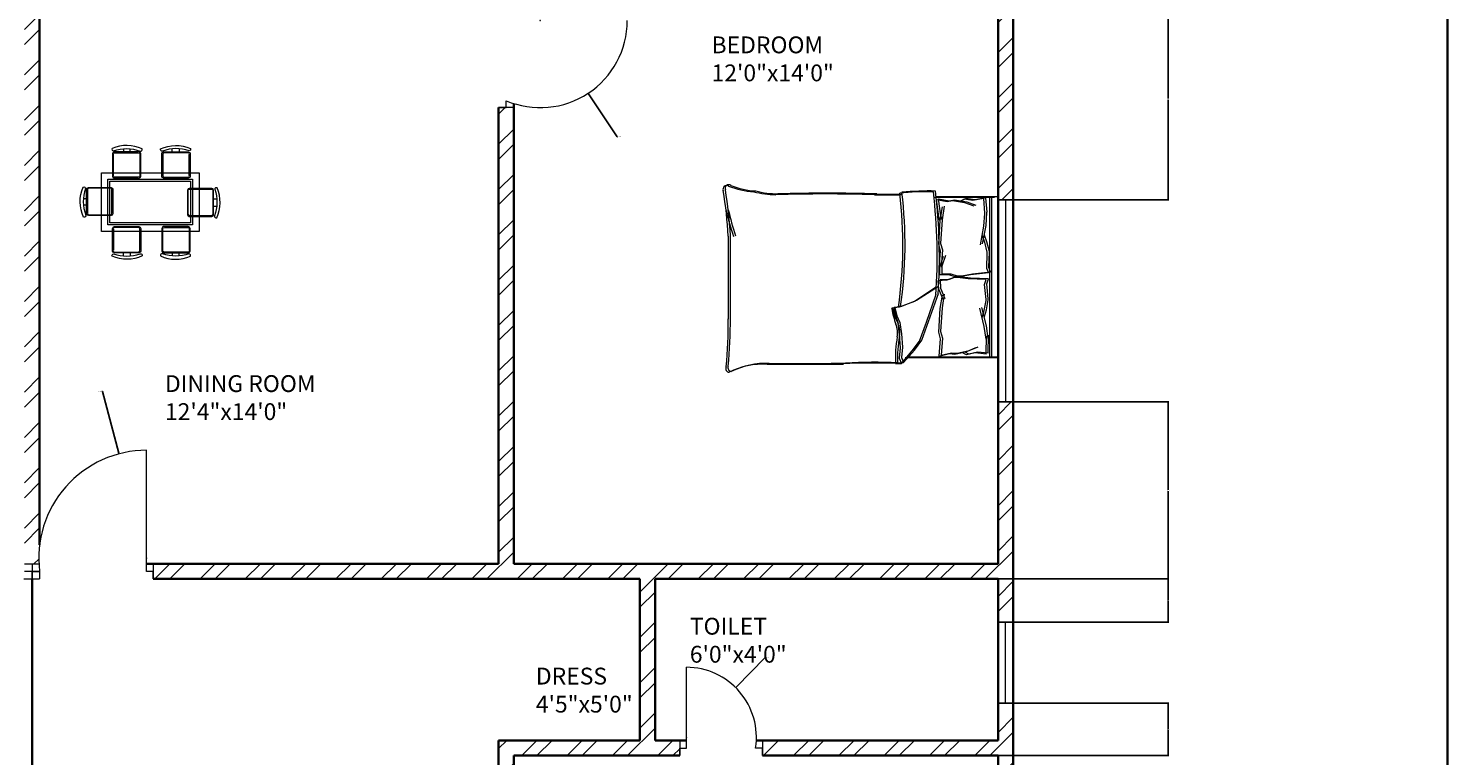
# Model space of a CAD drawing. Units: inches. Extents: x 392 to 1254, y 1207 to 2665.
# Tile 12 of 15: x 832 to 1254, y 1827 to 2043. Entities that reach past the tile are written whole.
import ezdxf

# ---------------------------------------------------------------- set-up
doc = ezdxf.new("R2010")
doc.units = ezdxf.units.IN
for name, color, linetype, lineweight in [('A-ANNO-DIMS', 2, 'Continuous', 18), ('A-ANNO-TTLB', 7, 'Continuous', 35), ('A-AREA-IDEN', 7, 'Continuous', 18), ('A-DOOR', 3, 'Continuous', 18), ('A-FURN', 8, 'Continuous', 13), ('A-GLAZ', 4, 'Continuous', 18), ('A-WALL', 7, 'Continuous', 35), ('A-WALL-PATT', 252, 'Continuous', 13)]:
    doc.layers.add(name, color=color, linetype=linetype, lineweight=lineweight)
doc.styles.get("Standard").update_dxf_attribs({"font": 'arial.ttf'})
doc.dimstyles.get("Standard").update_dxf_attribs({"dimtxt": 0.18, "dimasz": 0.18, "dimexe": 0.18, "dimexo": 0.0625, "dimgap": 0.09, "dimtad": 0, "dimtih": 1, "dimtoh": 1, "dimdec": 4, "dimzin": 0, "dimdsep": 46, "dimtxsty": 'Standard', "dimcen": 0.09, "dimadec": 0, "dimazin": 0, "dimtfac": 1, "dimtdec": 4, "dimtofl": 0, "dimtmove": 0, "dimatfit": 3, "dimfxl": 1, "dimtolj": 1, "dimtzin": 0, "dimarcsym": 0})

# ---------------------------------------------------------------- blocks, each defined once
blk = doc.blocks.new('BED-DOUBLE')
for p, q in [((3.47, 63.33), (3.47, 81.44)), ((3.48, 63.33), (3.48, 81.44)), ((3.7, 62.69), (3.7, 80.8)), ((3.7, 62.69), (3.7, 80.8)), ((51.27, 81.44), (51.27, 54.83)), ((51.27, 81.44), (51.27, 54.83)), ((51.49, 81.44), (51.49, 80.8)), ((51.49, 80.8), (51.49, 54.19)), ((51.49, 80.8), (51.49, 54.19)), ((3.47, 79.91), (51.27, 79.91)), ((3.48, 79.91), (51.27, 79.91)), ((3.7, 79.27), (51.49, 79.27)), ((3.7, 79.27), (51.49, 79.27)), ((3.89, 78.13), (4.47, 74.95)), ((3.89, 78.13), (4.47, 74.95)), ((3.9, 78.1), (8.18, 78.43)), ((3.9, 78.1), (8.18, 78.43)), ((4.12, 77.49), (4.7, 74.31)), ((4.12, 77.49), (4.7, 74.31)), ((4.13, 77.47), (8.41, 77.79)), ((4.13, 77.47), (8.41, 77.79)), ((8.18, 78.43), (8.28, 78.42)), ((8.18, 78.43), (8.28, 78.42)), ((8.28, 78.42), (12.11, 78.13)), ((8.28, 78.42), (12.11, 78.13)), ((8.41, 77.79), (8.51, 77.78)), ((8.41, 77.79), (8.51, 77.78)), ((8.51, 77.78), (12.34, 77.49)), ((8.51, 77.78), (12.34, 77.49)), ((12.11, 78.13), (17.6, 77.11)), ((12.11, 78.13), (17.6, 77.11)), ((12.34, 77.49), (17.83, 76.48)), ((12.34, 77.49), (17.83, 76.48)), ((14.85, 77.69), (16.88, 78.42)), ((14.85, 77.69), (16.88, 78.42)), ((15.08, 77.05), (17.11, 77.78)), ((15.08, 77.05), (17.11, 77.78)), ((16.88, 78.42), (19.77, 79.14)), ((16.88, 78.42), (19.77, 79.14)), ((17.11, 77.78), (20, 78.5)), ((17.11, 77.78), (20, 78.5)), ((19.77, 79.14), (20.09, 79.14)), ((19.77, 79.14), (20.09, 79.14)), ((20, 78.5), (20.32, 78.5)), ((20, 78.5), (20.32, 78.5)), ((20.09, 79.14), (24.54, 78.99)), ((20.09, 79.14), (24.54, 78.99)), ((20.32, 78.5), (24.77, 78.35)), ((20.32, 78.5), (24.77, 78.35)), ((24.54, 78.99), (25.98, 79.57)), ((24.54, 78.99), (25.98, 79.57)), ((24.77, 78.35), (26.21, 78.93)), ((24.77, 78.35), (26.21, 78.93)), ((25.98, 79.57), (26.56, 74.22)), ((25.98, 79.57), (26.56, 74.22)), ((26.21, 78.93), (26.79, 73.58)), ((26.21, 78.93), (26.79, 73.58)), ((27.98, 78.95), (27.73, 73.58)), ((27.98, 78.95), (27.73, 73.58)), ((28.21, 78.31), (27.96, 72.94)), ((28.21, 78.31), (27.96, 72.94)), ((29.46, 78.46), (27.98, 78.95)), ((29.46, 78.46), (27.98, 78.95)), ((29.68, 77.82), (28.21, 78.31)), ((29.68, 77.82), (28.21, 78.31)), ((33.88, 78.89), (29.46, 78.46)), ((33.88, 78.89), (29.46, 78.46)), ((34.11, 78.25), (29.68, 77.82)), ((34.11, 78.25), (29.68, 77.82)), ((34.2, 78.91), (33.88, 78.89)), ((34.2, 78.91), (33.88, 78.89)), ((34.43, 78.27), (34.11, 78.25)), ((34.43, 78.27), (34.11, 78.25)), ((37.14, 78.36), (34.2, 78.91)), ((37.14, 78.36), (34.2, 78.91)), ((37.36, 77.73), (34.43, 78.27)), ((37.36, 77.73), (34.43, 78.27)), ((41.91, 78.37), (36.49, 77.02)), ((41.91, 78.37), (36.5, 77.02)), ((42.14, 77.73), (36.72, 76.38)), ((42.14, 77.73), (36.72, 76.38)), ((39.2, 77.77), (37.14, 78.36)), ((39.2, 77.77), (37.14, 78.36)), ((39.43, 77.13), (37.36, 77.73)), ((39.43, 77.13), (37.36, 77.73)), ((45.71, 78.9), (41.91, 78.37)), ((45.71, 78.9), (41.91, 78.37)), ((45.94, 78.26), (42.14, 77.73)), ((45.94, 78.26), (42.14, 77.73)), ((50.11, 78.89), (44.71, 78.98)), ((44.71, 78.98), (45.71, 78.9)), ((50.11, 78.89), (44.71, 78.98)), ((44.71, 78.98), (45.71, 78.9)), ((50.34, 78.25), (44.94, 78.34)), ((44.94, 78.34), (45.94, 78.26)), ((50.34, 78.25), (44.94, 78.34)), ((44.94, 78.34), (45.94, 78.26)), ((50.11, 78.89), (49.73, 75.67)), ((50.11, 78.89), (49.73, 75.67)), ((50.34, 78.25), (49.96, 75.04)), ((50.34, 78.25), (49.96, 75.04)), ((4.47, 74.95), (4.04, 72.34)), ((4.47, 74.95), (4.04, 72.34)), ((4.04, 72.34), (4.62, 71.33)), ((4.04, 72.34), (4.62, 71.33)), ((4.7, 74.31), (4.27, 71.7)), ((4.7, 74.31), (4.27, 71.7)), ((4.47, 68.87), (5.05, 72.49)), ((4.47, 68.87), (5.05, 72.49)), ((4.7, 68.23), (5.28, 71.85)), ((4.7, 68.23), (5.28, 71.85)), ((5.05, 72.49), (6.06, 75.23)), ((5.05, 72.49), (6.06, 75.23)), ((5.28, 71.85), (6.29, 74.6)), ((5.28, 71.85), (6.29, 74.6)), ((26.56, 74.22), (27.14, 71.04)), ((26.56, 74.22), (27.14, 71.04)), ((26.79, 73.58), (27.37, 70.4)), ((26.79, 73.58), (27.37, 70.4)), ((27.73, 73.58), (27.35, 70.36)), ((27.73, 73.58), (27.35, 70.36)), ((27.96, 72.94), (27.58, 69.73)), ((27.96, 72.94), (27.58, 69.73)), ((49.31, 73.19), (48.13, 75.86)), ((49.31, 73.19), (48.13, 75.86)), ((49.54, 72.55), (48.36, 75.22)), ((49.54, 72.55), (48.36, 75.22)), ((50.11, 69.61), (49.31, 73.19)), ((50.11, 69.61), (49.31, 73.19)), ((50.34, 68.97), (49.54, 72.55)), ((50.34, 68.97), (49.54, 72.55)), ((49.73, 75.67), (50.33, 73.1)), ((49.73, 75.67), (50.33, 73.1)), ((50.33, 73.1), (49.81, 72.06)), ((50.33, 73.1), (49.81, 72.06)), ((49.96, 75.04), (50.56, 72.47)), ((49.96, 75.04), (50.56, 72.47)), ((50.56, 72.47), (50.04, 71.42)), ((50.56, 72.47), (50.04, 71.42)), ((4.27, 71.7), (4.85, 70.69)), ((4.27, 71.7), (4.85, 70.69)), ((4.76, 67.28), (4.47, 68.87)), ((4.76, 67.28), (4.47, 68.87)), ((4.99, 66.64), (4.7, 68.23)), ((4.99, 66.64), (4.7, 68.23)), ((27.14, 69.74), (26.56, 67.86)), ((27.14, 69.74), (26.56, 67.86)), ((26.56, 67.86), (26.56, 65.18)), ((26.56, 67.86), (26.56, 65.18)), ((27.37, 69.1), (26.79, 67.22)), ((27.37, 69.1), (26.79, 67.22)), ((27.14, 71.04), (27.14, 69.74)), ((27.14, 71.04), (27.14, 69.74)), ((27.35, 70.36), (27.44, 69.07)), ((27.35, 70.36), (27.44, 69.07)), ((27.37, 70.4), (27.37, 69.1)), ((27.37, 70.4), (27.37, 69.1)), ((27.44, 69.07), (28.13, 67.23)), ((27.44, 69.07), (28.13, 67.23)), ((27.58, 69.73), (27.66, 68.43)), ((27.58, 69.73), (27.66, 68.43)), ((27.66, 68.43), (28.36, 66.59)), ((27.66, 68.43), (28.36, 66.59)), ((49.92, 68.01), (50.11, 69.61)), ((49.92, 68.01), (50.11, 69.61)), ((50.7, 64.87), (49.92, 68.01)), ((50.7, 64.87), (49.92, 68.01)), ((50.15, 67.37), (50.34, 68.97)), ((50.15, 67.37), (50.34, 68.97)), ((4.18, 64.1), (4.76, 67.28)), ((4.18, 64.1), (4.76, 67.28)), ((9.28, 64.82), (4.18, 64.1)), ((9.28, 64.82), (4.18, 64.1)), ((4.41, 63.46), (4.99, 66.64)), ((4.41, 63.46), (4.99, 66.64)), ((9.51, 64.19), (4.41, 63.46)), ((9.51, 64.19), (4.41, 63.46)), ((6.38, 65.81), (10.41, 65.15)), ((6.38, 65.81), (10.41, 65.15)), ((6.61, 65.17), (10.64, 64.51)), ((6.61, 65.17), (10.64, 64.51)), ((10.41, 65.15), (9.28, 64.82)), ((10.41, 65.15), (9.28, 64.82)), ((10.64, 64.51), (9.51, 64.19)), ((10.64, 64.51), (9.51, 64.19)), ((10.41, 65.15), (17.42, 64.72)), ((10.41, 65.15), (17.42, 64.72)), ((10.64, 64.51), (17.65, 64.08)), ((10.64, 64.51), (17.65, 64.08)), ((17.42, 64.72), (19.38, 65.27)), ((17.42, 64.72), (19.38, 65.27)), ((17.65, 64.08), (19.61, 64.63)), ((17.65, 64.08), (19.61, 64.63)), ((19.38, 65.27), (24.52, 64.87)), ((19.38, 65.27), (24.52, 64.87)), ((19.61, 64.63), (24.74, 64.23)), ((19.61, 64.63), (24.74, 64.23)), ((24.1, 65.18), (20.96, 66.27)), ((24.1, 65.18), (20.96, 66.27)), ((24.33, 64.54), (21.19, 65.63)), ((24.33, 64.54), (21.19, 65.63)), ((26.56, 65.18), (24.1, 65.18)), ((26.56, 65.18), (24.1, 65.18)), ((26.79, 64.54), (24.33, 64.54)), ((26.79, 64.54), (24.33, 64.54)), ((26.79, 67.22), (26.79, 64.54)), ((26.79, 67.22), (26.79, 64.54)), ((28.13, 67.23), (28.3, 64.55)), ((28.13, 67.23), (28.3, 64.55)), ((28.3, 64.55), (30.75, 64.7)), ((28.3, 64.55), (30.75, 64.7)), ((28.36, 66.59), (28.53, 63.91)), ((28.36, 66.59), (28.53, 63.91)), ((28.53, 63.91), (30.98, 64.06)), ((28.53, 63.91), (30.98, 64.06)), ((30.26, 64.06), (34.45, 57.57)), ((30.26, 64.06), (34.45, 57.57)), ((30.49, 63.42), (34.68, 56.93)), ((30.49, 63.42), (34.68, 56.93)), ((30.75, 64.7), (33.82, 65.99)), ((30.75, 64.7), (33.82, 65.99)), ((30.98, 64.06), (34.05, 65.35)), ((30.98, 64.06), (34.05, 65.35)), ((40.64, 61.13), (32.31, 64.06)), ((40.64, 61.13), (32.31, 64.06)), ((40.87, 60.49), (32.53, 63.42)), ((40.87, 60.49), (32.53, 63.42)), ((32.56, 65.81), (36.6, 65.15)), ((32.56, 65.81), (36.6, 65.15)), ((32.79, 65.17), (36.82, 64.51)), ((32.79, 65.17), (36.82, 64.51)), ((36.6, 65.15), (43.61, 64.72)), ((36.6, 65.15), (43.61, 64.72)), ((36.82, 64.51), (43.83, 64.08)), ((36.82, 64.51), (43.83, 64.08)), ((43.61, 64.72), (45.57, 65.27)), ((43.61, 64.72), (45.57, 65.27)), ((43.83, 64.08), (45.79, 64.63)), ((43.83, 64.08), (45.79, 64.63)), ((45.57, 65.27), (50.7, 64.87)), ((45.57, 65.27), (50.7, 64.87)), ((45.79, 64.63), (50.93, 64.23)), ((45.79, 64.63), (50.93, 64.23)), ((50.93, 64.23), (50.15, 67.37)), ((50.93, 64.23), (50.15, 67.37)), ((46.22, 59.11), (40.64, 61.13)), ((46.22, 59.11), (40.64, 61.13)), ((46.45, 58.47), (40.87, 60.49)), ((46.45, 58.47), (40.87, 60.49)), ((49.16, 56.95), (46.22, 59.11)), ((49.16, 56.95), (46.22, 59.11)), ((34.45, 57.57), (36.15, 53.08)), ((34.45, 57.57), (36.15, 53.08)), ((34.68, 56.93), (36.38, 52.44)), ((34.68, 56.93), (36.38, 52.44)), ((49.39, 56.31), (46.45, 58.47)), ((49.39, 56.31), (46.45, 58.47)), ((52.87, 53.7), (49.16, 56.95)), ((52.87, 53.7), (49.16, 56.95)), ((53.1, 53.06), (49.39, 56.31)), ((53.1, 53.06), (49.39, 56.31)), ((36.15, 53.08), (36.46, 51.07)), ((36.15, 53.08), (36.46, 51.07)), ((36.38, 52.44), (36.69, 50.43)), ((36.38, 52.44), (36.69, 50.43)), ((36.46, 51.07), (38.94, 51.68)), ((36.46, 51.07), (38.94, 51.68)), ((36.69, 50.43), (39.17, 51.05)), ((36.69, 50.43), (39.17, 51.05)), ((38.94, 51.68), (40.95, 52.61)), ((38.94, 51.68), (40.95, 52.61)), ((39.17, 51.05), (41.18, 51.97)), ((39.17, 51.05), (41.18, 51.97)), ((40.95, 52.61), (44.36, 53.08)), ((40.95, 52.61), (44.36, 53.08)), ((41.18, 51.97), (44.59, 52.44)), ((41.18, 51.97), (44.59, 52.44)), ((44.36, 53.08), (48.23, 53.39)), ((44.36, 53.08), (48.23, 53.39)), ((44.59, 52.44), (48.46, 52.75)), ((44.59, 52.44), (48.46, 52.75)), ((48.23, 53.39), (51.33, 53.08)), ((48.23, 53.39), (51.33, 53.08)), ((48.46, 52.75), (51.56, 52.44)), ((48.46, 52.75), (51.56, 52.44)), ((51.33, 53.08), (52.87, 53.7)), ((51.33, 53.08), (52.87, 53.7)), ((51.56, 52.44), (53.1, 53.06)), ((51.56, 52.44), (53.1, 53.06)), ((52.95, 51.95), (52.87, 53.7, 3.87)), ((52.95, 51.95), (52.87, 53.7, 3.87)), ((53.18, 51.31), (53.1, 53.06, 3.87)), ((53.18, 51.31), (53.1, 53.06, 3.87)), ((15.06, 2.2), (39.68, 2.2)), ((15.06, 2.2), (39.68, 2.2)), ((15.29, 1.56), (39.91, 1.56)), ((15.29, 1.56), (39.91, 1.56))]:
    blk.add_line(p, q)
for centre, radius, start, end in [((21.36, -100.61), 164.97, 86.0865, 96.7821), ((21.36, -100.61), 164.97, 86.0865, 96.7821), ((21.59, -101.25), 164.97, 86.0865, 96.7821), ((21.59, -101.25), 164.97, 86.0865, 96.7821), ((85.16, 61.35), 83.31, 178.7218, 185.604), ((85.16, 61.35), 83.31, 178.7218, 185.604), ((85.39, 60.71), 83.31, 178.7218, 185.604), ((85.39, 60.71), 83.31, 178.7218, 185.604), ((17.76, -74.87), 129.02, 81.7845, 96.9006), ((17.76, -74.87), 129.02, 81.7845, 96.9006), ((17.98, -75.51), 129.02, 81.7845, 96.9006), ((17.98, -75.51), 129.02, 81.7845, 96.9006), ((-167.31, 50.27), 170.11, 358.4762, 1.0082), ((-167.31, 50.27), 170.11, 358.4762, 1.0082), ((-167.08, 49.63), 170.11, 358.4762, 1.0082), ((-167.08, 49.63), 170.11, 358.4762, 1.0082), ((36.64, 51), 0.185, 160.2464, 271.1377), ((36.64, 51), 0.185, 160.2464, 271.1377), ((31.15, 79.96), 29.65, 280.6617, 289.8806), ((31.15, 79.96), 29.65, 280.6617, 289.8806), ((31.38, 79.32), 29.65, 280.6617, 289.8806), ((31.38, 79.32), 29.65, 280.6617, 289.8806), ((43.74, 46.38), 6.22, 78.6608, 113.7384), ((43.74, 46.38), 6.22, 78.6608, 113.7384), ((43.97, 45.74), 6.22, 78.6608, 113.7384), ((43.97, 45.74), 6.22, 78.6608, 113.7384), ((51.33, 88.1), 36.18, 259.8763, 272.5657), ((51.33, 88.1), 36.18, 259.8763, 272.5657), ((51.56, 87.46), 36.18, 259.8763, 272.5657), ((51.56, 87.46), 36.18, 259.8763, 272.5657), ((182.27, 45.13), 129.5, 176.9791, 183.8365), ((182.27, 45.13), 129.5, 176.9791, 183.8365), ((182.49, 44.49), 129.5, 176.9791, 183.8365), ((182.49, 44.49), 129.5, 176.9791, 183.8365), ((36.86, 50.36), 0.185, 160.2464, 271.1377), ((36.86, 50.36), 0.185, 160.2464, 271.1377), ((484.82, 30.83), 482.31, 178.2277, 181.7185), ((484.82, 30.83), 482.31, 178.2277, 181.7185), ((485.05, 30.19), 482.31, 178.2277, 181.7185), ((485.05, 30.19), 482.31, 178.2277, 181.7185), ((-4508.74, 13.62), 4561.86, 0.00217, 0.28689), ((-4508.74, 13.62), 4561.86, 0.00217, 0.28689), ((-4508.51, 12.98), 4561.86, 0.00217, 0.28689), ((-4508.52, 12.98), 4561.86, 0.00217, 0.28689), ((-26.9, 16.93), 29.63, 346.0648, 358.9113), ((-26.9, 16.93), 29.63, 346.0648, 358.9113), ((-26.67, 16.29), 29.63, 346.0648, 358.9113), ((-26.67, 16.29), 29.63, 346.0648, 358.9113), ((76.16, 12.78), 23.07, 177.4714, 206.4681), ((76.16, 12.78), 23.07, 177.4714, 206.4681), ((76.39, 12.14), 23.07, 177.4714, 206.4681), ((76.39, 12.14), 23.07, 177.4714, 206.4681), ((-21.66, 11.17), 23.56, 337.9751, 356.652), ((-21.66, 11.17), 23.56, 337.9751, 356.652), ((-21.43, 10.53), 23.56, 337.9751, 356.652), ((-21.43, 10.53), 23.56, 337.9751, 356.652), ((1.09, 1.72), 1.09, 146.1736, 293.4781), ((1.09, 1.72), 1.09, 146.1736, 293.4781), ((1.32, 1.09), 1.09, 146.1736, 293.4781), ((1.32, 1.09), 1.09, 146.1736, 293.4781), ((21.43, -119.39), 121.76, 92.9958, 99.4091), ((21.43, -119.39), 121.76, 92.9958, 99.4091), ((21.66, -120.03), 121.76, 92.9958, 99.4091), ((21.65, -120.03), 121.76, 92.9958, 99.4091), ((-17.22, 105.15), 106.46, 283.3832, 287.7053), ((-17.22, 105.15), 106.46, 283.3832, 287.7053), ((-16.99, 104.52), 106.46, 283.3832, 287.7053), ((-16.99, 104.52), 106.46, 283.3832, 287.7053), ((41.15, -130.83), 133.04, 84.4998, 90.6351), ((41.15, -130.83), 133.04, 84.4998, 90.6351), ((41.38, -131.47), 133.04, 84.4998, 90.6351), ((41.38, -131.47), 133.04, 84.4998, 90.6351), ((54.41, 2.57), 1.1, 242.6588, 356.02), ((54.41, 2.57), 1.1, 242.6588, 356.02), ((54.64, 1.93), 1.1, 242.6588, 356.02), ((54.64, 1.93), 1.1, 242.6588, 356.02)]:
    blk.add_arc(centre, radius, start, end)
blk = doc.blocks.new('TABLE-DINING-RECT')
for points in [[(0, 17.41), (29.01, 17.41), (29.01, 0), (0, 0)], [(0, 17.41), (29.01, 17.41), (29.01, 0), (0, 0)], [(1.93, 15.47), (27.08, 15.47), (27.08, 1.93), (1.93, 1.93)], [(1.93, 15.47), (27.08, 15.47), (27.08, 1.93), (1.93, 1.93)], [(2.51, 14.89), (26.5, 14.89), (26.5, 2.51), (2.51, 2.51)], [(2.51, 14.89), (26.5, 14.89), (26.5, 2.51), (2.51, 2.51)]]:
    blk.add_lwpolyline(points, close=True)
blk = doc.blocks.new('WIN-60-A')
for p, q in [((0, 60), (4.5, 60)), ((4.5, 60), (2.25, 60)), ((2.25, 60), (2.25, 0)), ((2.25, 0), (0, 0)), ((0, 0), (4.5, 0))]:
    blk.add_line(p, q)
blk = doc.blocks.new('WIN-24-B')
for p, q in [((2.25, 24), (0, 24)), ((0, 24), (4.5, 24)), ((2.25, 0), (2.25, 24)), ((0, 0), (4.5, 0)), ((4.5, 0), (2.25, 0))]:
    blk.add_line(p, q)
blk = doc.blocks.new('*D32')
at = {"layer": 'A-ANNO-DIMS', "color": 0, "lineweight": -2, "transparency": 16777216}
for p, q in [((1120.34, 1842.92), (1171.06, 1842.92)), ((1170.88, 1842.74), (1170.88, 1835.29)), ((1170.88, 1827.48), (1170.88, 1834.93)), ((1120.34, 1827.3), (1171.06, 1827.3))]:
    blk.add_line(p, q, dxfattribs=at)
at = {"layer": 'A-ANNO-DIMS', "color": 0, "transparency": 16777216}
for points in [[(1170.85, 1842.74), (1170.91, 1842.74), (1170.88, 1842.92)], [(1170.85, 1827.48), (1170.91, 1827.48), (1170.88, 1827.3)]]:
    blk.add_solid(points, dxfattribs=at)
at = {"layer": 'Defpoints', "color": 0, "transparency": 16777216}
for p in [(1120.28, 1842.92), (1170.88, 1842.92), (1120.28, 1827.3)]:
    blk.add_point(p, dxfattribs=at)
at = {"layer": 'A-ANNO-DIMS', "color": 0, "transparency": 16777216, "insert": (1170.88, 1835.11), "char_height": 0.18, "attachment_point": 5}
blk.add_mtext('\\A1;15.624', dxfattribs=at)
blk = doc.blocks.new('*D33')
at = {"layer": 'A-ANNO-DIMS', "color": 0, "lineweight": -2, "transparency": 16777216}
for p, q in [((1120.34, 1932.46), (1171.06, 1932.46)), ((1170.88, 1932.28), (1170.88, 1906.31)), ((1170.88, 1879.98), (1170.88, 1905.94)), ((1120.34, 1879.8), (1171.06, 1879.8))]:
    blk.add_line(p, q, dxfattribs=at)
at = {"layer": 'A-ANNO-DIMS', "color": 0, "transparency": 16777216}
for points in [[(1170.85, 1932.28), (1170.91, 1932.28), (1170.88, 1932.46)], [(1170.85, 1879.98), (1170.91, 1879.98), (1170.88, 1879.8)]]:
    blk.add_solid(points, dxfattribs=at)
at = {"layer": 'Defpoints', "color": 0, "transparency": 16777216}
for p in [(1120.28, 1932.46), (1170.88, 1932.46), (1120.28, 1879.8)]:
    blk.add_point(p, dxfattribs=at)
at = {"layer": 'A-ANNO-DIMS', "color": 0, "transparency": 16777216, "insert": (1170.88, 1906.13), "char_height": 0.18, "attachment_point": 5}
blk.add_mtext('\\A1;52.66', dxfattribs=at)
blk = doc.blocks.new('*D40')
at = {"layer": 'A-ANNO-DIMS', "color": 0, "lineweight": -2, "transparency": 16777216}
for p, q in [((1120.34, 2052.3), (1171.06, 2052.3)), ((1170.88, 2052.12), (1170.88, 2022.56)), ((1170.88, 1992.64), (1170.88, 2022.19)), ((1120.34, 1992.46), (1171.06, 1992.46))]:
    blk.add_line(p, q, dxfattribs=at)
at = {"layer": 'A-ANNO-DIMS', "color": 0, "transparency": 16777216}
for points in [[(1170.85, 2052.12), (1170.91, 2052.12), (1170.88, 2052.3)], [(1170.85, 1992.64), (1170.91, 1992.64), (1170.88, 1992.46)]]:
    blk.add_solid(points, dxfattribs=at)
at = {"layer": 'Defpoints', "color": 0, "transparency": 16777216}
for p in [(1120.28, 2052.3), (1120.28, 1992.46), (1170.88, 1992.46)]:
    blk.add_point(p, dxfattribs=at)
at = {"layer": 'A-ANNO-DIMS', "color": 0, "transparency": 16777216, "insert": (1170.88, 2022.38), "char_height": 0.18, "attachment_point": 5}
blk.add_mtext('\\A1;59.84', dxfattribs=at)
blk = doc.blocks.new('*D41')
at = {"layer": 'A-ANNO-DIMS', "color": 0, "lineweight": -2, "transparency": 16777216}
for p, q in [((1120.34, 1879.8), (1171.06, 1879.8)), ((1170.88, 1879.62), (1170.88, 1873.54)), ((1170.88, 1867.1), (1170.88, 1873.18)), ((1120.34, 1866.92), (1171.06, 1866.92))]:
    blk.add_line(p, q, dxfattribs=at)
at = {"layer": 'A-ANNO-DIMS', "color": 0, "transparency": 16777216}
for points in [[(1170.85, 1879.62), (1170.91, 1879.62), (1170.88, 1879.8)], [(1170.85, 1867.1), (1170.91, 1867.1), (1170.88, 1866.92)]]:
    blk.add_solid(points, dxfattribs=at)
at = {"layer": 'Defpoints', "color": 0, "transparency": 16777216}
for p in [(1120.28, 1879.8), (1120.28, 1866.92), (1170.88, 1866.92)]:
    blk.add_point(p, dxfattribs=at)
at = {"layer": 'A-ANNO-DIMS', "color": 0, "transparency": 16777216, "insert": (1170.88, 1873.36), "char_height": 0.18, "attachment_point": 5}
blk.add_mtext('\\A1;12.876', dxfattribs=at)
blk = doc.blocks.new('*D84')
at = {"layer": 'A-ANNO-DIMS', "color": 0, "lineweight": -2, "transparency": 16777216}
for p, q in [((853.76, 1935.56), (853.94, 1935.56)), ((853.94, 1935.56), (858.83, 1917.15)), ((867, 1885.99), (867.18, 1885.99)), ((867.09, 1885.9), (867.09, 1886.08))]:
    blk.add_line(p, q, dxfattribs=at)
at = {"layer": 'A-ANNO-DIMS', "color": 0, "transparency": 16777216}
blk.add_solid([(858.86, 1917.16), (858.8, 1917.14), (858.87, 1916.97)], dxfattribs=at)
at = {"layer": 'Defpoints', "color": 0, "transparency": 16777216}
for p in [(858.87, 1916.97), (867.09, 1885.99)]:
    blk.add_point(p, dxfattribs=at)
at = {"layer": 'A-ANNO-DIMS', "color": 0, "transparency": 16777216, "insert": (853.21, 1935.56), "char_height": 0.18, "attachment_point": 5}
blk.add_mtext('\\A1;R32.054', dxfattribs=at)
blk = doc.blocks.new('*D96')
at = {"layer": 'A-ANNO-DIMS', "color": 0, "lineweight": -2, "transparency": 16777216}
for p, q in [((984.08, 2045.75), (984.26, 2045.75)), ((984.17, 2045.66), (984.17, 2045.84)), ((1006.98, 2011.23), (998.53, 2024.02)), ((1007.16, 2011.23), (1006.98, 2011.23))]:
    blk.add_line(p, q, dxfattribs=at)
at = {"layer": 'A-ANNO-DIMS', "color": 0, "transparency": 16777216}
blk.add_solid([(998.55, 2024.04), (998.5, 2024.01), (998.43, 2024.17)], dxfattribs=at)
at = {"layer": 'Defpoints', "color": 0, "transparency": 16777216}
for p in [(984.17, 2045.75), (998.43, 2024.17)]:
    blk.add_point(p, dxfattribs=at)
at = {"layer": 'A-ANNO-DIMS', "color": 0, "transparency": 16777216, "insert": (1007.71, 2011.23), "char_height": 0.18, "attachment_point": 5}
blk.add_mtext('\\A1;R25.864', dxfattribs=at)
blk = doc.blocks.new('*D102')
at = {"layer": 'A-ANNO-DIMS', "color": 0, "lineweight": -2, "transparency": 16777216}
for p, q in [((1051.03, 1856.44), (1042.37, 1847.67)), ((1051.21, 1856.44), (1051.03, 1856.44)), ((1027.53, 1832.72), (1027.71, 1832.72)), ((1027.62, 1832.63), (1027.62, 1832.81))]:
    blk.add_line(p, q, dxfattribs=at)
at = {"layer": 'A-ANNO-DIMS', "color": 0, "transparency": 16777216}
blk.add_solid([(1042.35, 1847.69), (1042.4, 1847.65), (1042.25, 1847.54)], dxfattribs=at)
at = {"layer": 'Defpoints', "color": 0, "transparency": 16777216}
for p in [(1042.25, 1847.54), (1027.62, 1832.72)]:
    blk.add_point(p, dxfattribs=at)
at = {"layer": 'A-ANNO-DIMS', "color": 0, "transparency": 16777216, "insert": (1051.76, 1856.44), "char_height": 0.18, "attachment_point": 5}
blk.add_mtext('\\A1;R20.826', dxfattribs=at)

msp = doc.modelspace()

# ---------------------------------------------------------------- hatches: boundary and pattern name
at = {"layer": 'A-WALL-PATT'}
h = msp.add_hatch(dxfattribs=at)
h.set_pattern_fill('ANSI32', color=256)
h.paths.add_polyline_path([(579.5309, 2227.0453), (579.5309, 2229.2953), (541.2807, 2229.2953), (541.2807, 2182.3091), (545.7807, 2182.3091), (545.7807, 2224.7953), (579.5309, 2224.7953)])
h.paths.add_polyline_path([(655.4442, 2229.2953), (627.5309, 2229.2953), (627.5309, 2224.7953), (655.4442, 2224.7953), (655.4442, 2227.0453)])
h.paths.add_polyline_path([(703.0758, 2229.2953), (678.5257, 2229.2953), (678.5257, 2227.0453), (678.5257, 2224.7953), (689.7807, 2224.7953), (689.7807, 2158.6973), (694.2807, 2158.6973), (694.2807, 2224.7953), (703.0758, 2224.7953)])
h.paths.add_polyline_path([(768.5767, 2229.2953), (727.0758, 2229.2953), (727.0758, 2224.7953), (742.2807, 2224.7953), (742.2807, 2128.7953), (694.2807, 2128.7953), (694.2807, 2134.0554), (689.7807, 2134.0554), (689.7807, 2090.2854), (694.2807, 2090.2854), (694.2807, 2124.2953), (742.2807, 2124.2953), (742.2807, 2052.2953), (795.2124, 2052.2953), (795.2124, 2054.5453), (795.2124, 2056.7953), (746.7807, 2056.7953), (746.7807, 2224.7953), (768.5767, 2224.7953)])
h.paths.add_polyline_path([(867.5089, 2229.2953), (804.5767, 2229.2953), (804.5767, 2224.7953), (830.7807, 2224.7953), (830.7807, 2056.7953), (826.9066, 2056.7953), (826.9066, 2052.2953), (830.7807, 2052.2953), (830.7807, 1886.6777, -0.01766664), (830.8602, 1884.2953), (835.0818, 1884.2953, -0.04411348), (835.2807, 1889.9369), (835.2807, 2052.2953), (839.418, 2052.2953), (839.418, 2056.7953), (835.2807, 2056.7953), (835.2807, 2224.7953), (867.5089, 2224.7953)])
h.paths.add_polyline_path([(939.8604, 2229.2953), (903.5089, 2229.2953), (903.5089, 2227.0453), (903.5089, 2224.7953), (919.2807, 2224.7953), (919.2807, 2056.7953), (870.6499, 2056.7953), (870.6499, 2052.2953), (923.7807, 2052.2953), (923.7807, 2124.2953), (971.7807, 2124.2953), (971.7807, 2089.7112), (974.0307, 2089.7112), (976.2807, 2089.7112), (976.2807, 2133.56), (974.0307, 2133.56), (971.7807, 2133.56), (971.7807, 2128.7953), (923.7807, 2128.7953), (923.7807, 2224.7953), (939.8604, 2224.7953)])
h.paths.add_polyline_path([(1124.7807, 2229.2953), (1009.403, 2229.2953), (1009.403, 2224.7953), (1120.2807, 2224.7953), (1120.2807, 2184.7605), (1124.7807, 2184.7605)])
h.paths.add_polyline_path([(1124.7807, 2124.7605), (1120.2807, 2124.7605), (1120.2807, 2056.7953), (976.2807, 2056.7953), (976.2807, 2061.471), (971.7807, 2061.471), (971.7807, 2047.7483), (974.0307, 2047.7483), (976.2807, 2047.7483), (976.2807, 2052.2953), (1120.2807, 2052.2953), (1120.2807, 1992.457), (1124.7807, 1992.457)])
h.paths.add_polyline_path([(1124.7807, 1932.457), (1122.5307, 1932.457), (1120.2807, 1932.457), (1120.2807, 1884.2953), (976.2807, 1884.2953), (976.2807, 2019.9536), (971.7807, 2019.9536), (971.7807, 1884.2953), (869.0911, 1884.2953), (869.0911, 1879.7953), (971.7807, 1879.7953), (1013.7807, 1879.7953), (1013.7807, 1831.7953), (971.7807, 1831.7953), (971.7807, 1822.3831), (974.0307, 1822.3831), (976.2807, 1822.3831), (976.2807, 1827.2953), (1013.7807, 1827.2953), (1025.6191, 1827.2953), (1025.6191, 1829.5453), (1025.6191, 1831.7953), (1018.2807, 1831.7953), (1018.2807, 1879.7953), (1120.2807, 1879.7953), (1120.2807, 1866.9192), (1124.7807, 1866.9192)])
h.paths.add_polyline_path([(1124.7807, 1842.9192), (1122.5307, 1842.9192), (1120.2807, 1842.9192), (1120.2807, 1831.7953), (1050.2021, 1831.7953), (1050.2021, 1827.2953), (1120.2807, 1827.2953), (1120.2807, 1781.4559), (1124.7807, 1781.4559)])
h.paths.add_polyline_path([(976.2807, 1790.8718), (971.7807, 1790.8718), (971.7807, 1648.3339), (976.2807, 1648.3339), (976.2807, 1654.7953), (1120.2807, 1654.7953), (1120.2807, 1626.3807), (1124.7807, 1626.3807), (1124.7807, 1721.4559), (1120.2807, 1721.4559), (1120.2807, 1659.2953), (976.2807, 1659.2953)])
h.paths.add_polyline_path([(1124.7807, 1566.3807), (1120.2807, 1566.3807), (1120.2807, 1486.7953), (1101.07, 1486.7953), (1101.07, 1482.2953), (1124.7807, 1482.2953)])
h.paths.add_polyline_path([(1041.07, 1484.5453), (1041.07, 1486.7953), (1006.2807, 1486.7953), (1006.2807, 1484.5453), (1006.2807, 1482.2953), (1041.07, 1482.2953)])
h.paths.add_polyline_path([(976.2807, 1617.5497), (974.0307, 1617.5497), (971.7807, 1617.5497), (971.7807, 1599.2953), (965.8041, 1599.2953), (965.8041, 1594.7953), (971.7807, 1594.7953), (971.7807, 1486.7953), (954.1249, 1486.7953), (954.1249, 1482.2953), (981.5717, 1482.2953), (981.5717, 1484.5453), (981.5717, 1486.7953), (976.2807, 1486.7953)])
h.paths.add_polyline_path([(930.1249, 1486.7953), (887.7807, 1486.7953), (887.7807, 1594.7953), (941.9141, 1594.7953), (941.9141, 1597.0453), (941.9141, 1599.2953), (887.7807, 1599.2953), (887.7807, 1659.2953), (863.5916, 1659.2953), (863.5916, 1654.7953), (883.2807, 1654.7953), (883.2807, 1438.7953), (782.7807, 1438.7953), (782.7807, 1486.7953), (782.7807, 1654.7953), (800.1309, 1654.7953), (800.1309, 1657.0453), (800.1309, 1659.2953), (778.2807, 1659.2953), (778.2807, 1599.2953), (721.7333, 1599.2953), (721.7333, 1597.0453), (721.7333, 1594.7953), (778.2807, 1594.7953), (778.2807, 1486.7953), (729.598, 1486.7953), (729.598, 1482.2953), (753.2885, 1482.2953), (753.2885, 1410.2953), (922.9852, 1410.2953), (922.9852, 1482.2953), (930.1249, 1482.2953)])
h.paths.add_polyline_path([(918.4852, 1482.2953), (918.4852, 1414.7953), (757.7885, 1414.7953), (757.7885, 1482.2953), (778.2807, 1482.2953), (778.2807, 1434.2953), (782.7807, 1434.2953), (887.7807, 1434.2953), (887.7807, 1438.7953), (887.7807, 1482.2953)], flags=16)
h.paths.add_polyline_path([(694.2807, 1594.7953), (700.4169, 1594.7953), (700.4169, 1597.0453), (700.4169, 1599.2953), (694.2807, 1599.2953), (694.2807, 1617.7503), (692.0307, 1617.7503), (689.7807, 1617.7503), (689.7807, 1486.7953), (682.7672, 1486.7953), (682.7672, 1482.2953), (705.598, 1482.2953), (705.598, 1484.5453), (705.598, 1486.7953), (694.2807, 1486.7953)])
h.paths.add_polyline_path([(545.7807, 1654.7953), (689.7807, 1654.7953), (689.7807, 1649.7691), (694.2807, 1649.7691), (694.2807, 1789.3981), (692.0307, 1789.3981), (689.7807, 1789.3981), (689.7807, 1659.2953), (545.7807, 1659.2953), (545.7807, 1714.4681), (543.5307, 1714.4681), (541.2807, 1714.4681), (541.2807, 1482.2953), (567.0628, 1482.2953), (567.0628, 1484.5453), (567.0628, 1486.7953), (545.7807, 1486.7953)])
h.paths.add_polyline_path([(545.7807, 1827.2953), (620.2247, 1827.2953), (620.2247, 1829.5453), (620.2247, 1831.7953), (545.7807, 1831.7953), (545.7807, 1846.8518), (541.2807, 1846.8518), (541.2807, 1774.4681), (545.7807, 1774.4681)])
h.paths.add_polyline_path([(797.0944, 1884.2953), (694.2807, 1884.2953), (694.2807, 2019.0288), (692.0307, 2019.0288), (689.7807, 2019.0288), (689.7807, 1884.2953), (545.7807, 1884.2953), (545.7807, 1951.8244), (541.2807, 1951.8244), (541.2807, 1870.8518), (543.5307, 1870.8518), (545.7807, 1870.8518), (545.7807, 1879.7953), (647.7807, 1879.7953), (647.7807, 1831.7953), (642.6413, 1831.7953), (642.6413, 1827.2953), (652.2807, 1827.2953), (689.7807, 1827.2953), (689.7807, 1821.0531), (694.2807, 1821.0531), (694.2807, 1831.7953), (652.2807, 1831.7953), (652.2807, 1879.7953), (797.0944, 1879.7953), (797.0944, 1882.0453)])
h.paths.add_polyline_path([(545.7807, 2122.3091), (541.2807, 2122.3091), (541.2807, 2011.8244), (543.5307, 2011.8244), (545.7807, 2011.8244), (545.7807, 2052.2953), (689.7807, 2052.2953), (689.7807, 2048.2048), (694.2807, 2048.2048), (694.2807, 2061.3129), (692.0307, 2061.3129), (689.7807, 2061.3129), (689.7807, 2056.7953), (545.7807, 2056.7953)])

# ---------------------------------------------------------------- linework, layer by layer
at = {"layer": 'A-ANNO-TTLB'}
msp.add_lwpolyline([(391.939, 2664.8979), (1253.97, 2664.8979), (1253.97, 1207.2611), (391.939, 1207.2611)], close=True, dxfattribs=at)
at = {"layer": 'A-DOOR'}
for p, q in [((974.0307, 2019.9536), (974.0307, 2021.9536)), ((976.2807, 2019.9536), (971.7807, 2019.9536)), ((971.7807, 2019.9536), (974.0307, 2019.9536)), ((867.0911, 1882.0453), (867.0911, 1918.0453)), ((830.7807, 1884.2953), (835.0818, 1884.2953)), ((833.0352, 1884.2953), (833.0352, 1879.7953)), ((869.0911, 1884.2953), (869.0911, 1879.7953)), ((830.5499, 1879.7953), (835.2807, 1879.7953)), ((833.0352, 1882.0453), (830.7807, 1882.0453)), ((833.0352, 1879.7953), (833.0352, 1882.0453)), ((833.0352, 1882.0453), (835.2807, 1882.0453)), ((835.2807, 1882.0453), (833.0352, 1882.0453)), ((835.2807, 1882.0453), (835.2807, 1879.7953)), ((869.0911, 1882.0453), (867.0911, 1882.0453)), ((869.0911, 1879.7953), (869.0911, 1882.0453)), ((1027.6191, 1829.5453), (1027.6191, 1853.5453)), ((1025.6191, 1831.7953), (1025.6191, 1827.2953)), ((1050.2021, 1831.7953), (1050.2021, 1827.2953)), ((1025.6191, 1827.2953), (1025.6191, 1829.5453)), ((1025.6191, 1829.5453), (1027.6191, 1829.5453)), ((1050.2021, 1829.5453), (1048.2021, 1829.5453)), ((1050.2021, 1827.2953), (1050.2021, 1829.5453))]:
    msp.add_line(p, q, dxfattribs=at)
for centre, radius, start, end in [((984.167, 2045.7483), 25.8637, 246.92657, 0), ((867.0911, 1885.9911), 32.0542, 90, 187.070916), ((1027.6191, 1832.719), 20.8263, 351.234633, 90)]:
    msp.add_arc(centre, radius, start, end, dxfattribs=at)
at = {"layer": 'A-FURN'}
for points in [[(857.2729, 2007.0442, -0.17580919), (865.1746, 2006.9844, 0.57839206), (865.7732, 2007.6426, 0.21452438), (856.8539, 2007.7623, 0.55201397), (857.2729, 2007.0442, -0.06507904)], [(857.2729, 2007.0439, -0.17580919), (865.1746, 2006.9841, 0.57839206), (865.7732, 2007.6423, 0.21452438), (856.8539, 2007.762, 0.55201397), (857.2729, 2007.0439, -0.06507904)], [(864.8394, 2006.7271), (857.5037, 2006.7271, 0.41421356), (856.9905, 2006.2139), (856.9905, 1999.4689, 0.41421356), (857.5037, 1998.9556), (864.8394, 1998.9556, 0.41421356), (865.3526, 1999.4689), (865.3526, 2006.2139, 0.41421356), (864.8394, 2006.7271)], [(864.8394, 2006.7268), (857.5037, 2006.7268, 0.41421356), (856.9905, 2006.2136), (856.9905, 1999.4685, 0.41421356), (857.5037, 1998.9553), (864.8394, 1998.9553, 0.41421356), (865.3526, 1999.4685), (865.3526, 2006.2136, 0.41421356), (864.8394, 2006.7268)], [(862.2627, 2006.7271), (862.2627, 2007.6548, -0.06475861)], [(862.2627, 2006.7268), (862.2627, 2007.6545, -0.06475861)], [(871.8268, 2006.9844, -0.57839206), (871.2282, 2007.6426, -0.21452438), (880.1476, 2007.7623, -0.55201397), (879.7285, 2007.0442, 0.1758092), (871.8268, 2006.9844)], [(871.8268, 2006.9841, -0.57839206), (871.2282, 2007.6423, -0.21452438), (880.1476, 2007.762, -0.55201397), (879.7285, 2007.0439, 0.1758092), (871.8268, 2006.9841)], [(879.4977, 2006.7271, -0.41421356), (880.0109, 2006.2139), (880.0109, 1999.4689, -0.41421356), (879.4977, 1998.9556), (872.1621, 1998.9556, -0.41421356), (871.6488, 1999.4689), (871.6488, 2006.2139, -0.41421356), (872.1621, 2006.7271), (879.4977, 2006.7271)], [(879.4977, 2006.7268, -0.41421356), (880.011, 2006.2136), (880.011, 1999.4685, -0.41421356), (879.4977, 1998.9553), (872.1621, 1998.9553, -0.41421356), (871.6489, 1999.4685), (871.6489, 2006.2136, -0.41421356), (872.1621, 2006.7268), (879.4977, 2006.7268)], [(874.7387, 2006.7271), (874.7387, 2007.6548, 0.06475861)], [(874.7387, 2006.7268), (874.7387, 2007.6545, 0.06475861)], [(849.0062, 1987.9628, -0.57839206), (848.348, 1987.3642, -0.21452438), (848.2283, 1996.2835, -0.55201397), (848.9464, 1995.8645, 0.17580937), (849.0062, 1987.9628)], [(849.0062, 1987.9625, -0.57839206), (848.348, 1987.3639, -0.21452438), (848.2283, 1996.2832, -0.55201397), (848.9464, 1995.8642, 0.17580937), (849.0062, 1987.9625)], [(849.2635, 1995.6337, -0.41421356), (849.7767, 1996.1469), (856.5217, 1996.1469, -0.41421356), (857.0349, 1995.6337), (857.0349, 1988.298, -0.41421356), (856.5217, 1987.7848), (849.7767, 1987.7848, -0.41421356), (849.2635, 1988.298), (849.2635, 1995.6337)], [(849.2635, 1995.6334, -0.41421356), (849.7767, 1996.1466), (856.5217, 1996.1466, -0.41421356), (857.035, 1995.6334), (857.035, 1988.2977, -0.41421356), (856.5217, 1987.7845), (849.7767, 1987.7845, -0.41421356), (849.2635, 1988.2977), (849.2635, 1995.6334)], [(887.0388, 1995.3825, 0.41421356), (886.5256, 1995.8957), (879.7806, 1995.8957, 0.41421356), (879.2674, 1995.3825), (879.2674, 1988.0468, 0.41421356), (879.7806, 1987.5336), (886.5256, 1987.5336, 0.41421356), (887.0388, 1988.0468), (887.0388, 1995.3825)], [(887.0388, 1995.3822, 0.41421356), (886.5256, 1995.8954), (879.7806, 1995.8954, 0.41421356), (879.2674, 1995.3822), (879.2674, 1988.0465, 0.41421356), (879.7806, 1987.5333), (886.5256, 1987.5333, 0.41421356), (887.0388, 1988.0465), (887.0388, 1995.3822)], [(887.3559, 1995.6133, -0.17580919), (887.2961, 1987.7116, 0.57839206), (887.9543, 1987.113, 0.21452438), (888.074, 1996.0323, 0.55201397), (887.3559, 1995.6133, -0.06507904)], [(887.3559, 1995.613, -0.17580919), (887.2961, 1987.7113, 0.57839206), (887.9543, 1987.1126, 0.21452438), (888.074, 1996.032, 0.55201397), (887.3559, 1995.613, -0.06507904)], [(849.2635, 1990.8747), (848.3358, 1990.8747, 0.06475861)], [(849.2635, 1990.8744), (848.3358, 1990.8744, 0.06475861)], [(887.0388, 1990.6235), (887.9665, 1990.6235, -0.06475861)], [(887.0388, 1990.6232), (887.9665, 1990.6232, -0.06475861)], [(864.8394, 1976.7439), (857.5037, 1976.7439, -0.41421356), (856.9905, 1977.2571), (856.9905, 1984.0021, -0.41421356), (857.5037, 1984.5153), (864.8394, 1984.5153, -0.41421356), (865.3526, 1984.0021), (865.3526, 1977.2571, -0.41421356), (864.8394, 1976.7439)], [(864.8394, 1976.7435), (857.5037, 1976.7435, -0.41421356), (856.9905, 1977.2568), (856.9905, 1984.0018, -0.41421356), (857.5037, 1984.515), (864.8394, 1984.515, -0.41421356), (865.3526, 1984.0018), (865.3526, 1977.2568, -0.41421356), (864.8394, 1976.7435)], [(879.4977, 1976.7439, 0.41421356), (880.0109, 1977.2571), (880.0109, 1984.0021, 0.41421356), (879.4977, 1984.5153), (872.1621, 1984.5153, 0.41421356), (871.6488, 1984.0021), (871.6488, 1977.2571, 0.41421356), (872.1621, 1976.7439), (879.4977, 1976.7439)], [(879.4977, 1976.7435, 0.41421356), (880.011, 1977.2568), (880.011, 1984.0018, 0.41421356), (879.4977, 1984.515), (872.1621, 1984.515, 0.41421356), (871.6489, 1984.0018), (871.6489, 1977.2568, 0.41421356), (872.1621, 1976.7435), (879.4977, 1976.7435)], [(865.1746, 1976.4866, -0.57839206), (865.7732, 1975.8283, -0.21452438), (856.8539, 1975.7087, -0.55201397), (857.2729, 1976.4267, 0.17580929), (865.1746, 1976.4866)], [(865.1746, 1976.4862, -0.57839206), (865.7732, 1975.828, -0.21452438), (856.8539, 1975.7083, -0.55201397), (857.2729, 1976.4264, 0.17580929), (865.1746, 1976.4862)], [(862.2627, 1976.7439), (862.2627, 1975.8161, 0.06475861)], [(862.2627, 1976.7435), (862.2627, 1975.8158, 0.06475861)], [(879.7285, 1976.4267, -0.17580928), (871.8268, 1976.4866, 0.57839206), (871.2282, 1975.8283, 0.21452438), (880.1476, 1975.7087, 0.55201397), (879.7285, 1976.4267, -0.06507904)], [(879.7285, 1976.4264, -0.17580928), (871.8268, 1976.4862, 0.57839206), (871.2282, 1975.828, 0.21452438), (880.1476, 1975.7083, 0.55201397), (879.7285, 1976.4264, -0.06507904)], [(874.7387, 1976.7439), (874.7387, 1975.8161, -0.06475861)], [(874.7387, 1976.7435), (874.7387, 1975.8158, -0.06475861)]]:
    msp.add_lwpolyline(points, format="xyb", dxfattribs=at)
for points in [[(857.5068, 2006.4959), (864.6082, 2006.4959, -0.41421356), (865.1214, 2005.9827), (865.1214, 1999.7001, -0.41421356), (864.6082, 1999.1868), (857.5068, 1999.1868, -0.51206948), (857.2217, 1999.7001), (857.2217, 2005.9827, -0.51206948)], [(857.5068, 2006.4956), (864.6082, 2006.4956, -0.41421356), (865.1214, 2005.9824), (865.1214, 1999.6998, -0.41421356), (864.6082, 1999.1865), (857.5068, 1999.1865, -0.51206948), (857.2217, 1999.6998), (857.2217, 2005.9824, -0.51206948)], [(879.4946, 2006.4959), (872.3933, 2006.4959, 0.41421356), (871.88, 2005.9827), (871.88, 1999.7001, 0.41421356), (872.3933, 1999.1868), (879.4946, 1999.1868, 0.51206948), (879.7797, 1999.7001), (879.7797, 2005.9827, 0.51206948)], [(879.4946, 2006.4956), (872.3933, 2006.4956, 0.41421356), (871.8801, 2005.9824), (871.8801, 1999.6998, 0.41421356), (872.3933, 1999.1865), (879.4946, 1999.1865, 0.51206948), (879.7797, 1999.6998), (879.7797, 2005.9824, 0.51206948)], [(849.4947, 1995.6306), (849.4947, 1988.5292, 0.41421356), (850.0079, 1988.016), (856.2905, 1988.016, 0.41421356), (856.8037, 1988.5292), (856.8037, 1995.6306, 0.51206948), (856.2905, 1995.9157), (850.0079, 1995.9157, 0.51206948)], [(849.4947, 1995.6303), (849.4947, 1988.5289, 0.41421356), (850.0079, 1988.0157), (856.2905, 1988.0157, 0.41421356), (856.8038, 1988.5289), (856.8038, 1995.6303, 0.51206948), (856.2905, 1995.9154), (850.0079, 1995.9154, 0.51206948)], [(886.8076, 1995.3794), (886.8076, 1988.278, -0.41421356), (886.2944, 1987.7648), (880.0118, 1987.7648, -0.41421356), (879.4986, 1988.278), (879.4986, 1995.3794, -0.51206948), (880.0118, 1995.6645), (886.2944, 1995.6645, -0.51206948)], [(886.8076, 1995.3791), (886.8076, 1988.2777, -0.41421356), (886.2944, 1987.7645), (880.0118, 1987.7645, -0.41421356), (879.4986, 1988.2777), (879.4986, 1995.3791, -0.51206948), (880.0118, 1995.6642), (886.2944, 1995.6642, -0.51206948)], [(857.5068, 1976.9751), (864.6082, 1976.9751, 0.41421356), (865.1214, 1977.4883), (865.1214, 1983.7709, 0.41421356), (864.6082, 1984.2841), (857.5068, 1984.2841, 0.51206948), (857.2217, 1983.7709), (857.2217, 1977.4883, 0.51206948)], [(857.5068, 1976.9748), (864.6082, 1976.9748, 0.41421356), (865.1214, 1977.488), (865.1214, 1983.7706, 0.41421356), (864.6082, 1984.2838), (857.5068, 1984.2838, 0.51206948), (857.2217, 1983.7706), (857.2217, 1977.488, 0.51206948)], [(879.4946, 1976.9751), (872.3933, 1976.9751, -0.41421356), (871.88, 1977.4883), (871.88, 1983.7709, -0.41421356), (872.3933, 1984.2841), (879.4946, 1984.2841, -0.51206948), (879.7797, 1983.7709), (879.7797, 1977.4883, -0.51206948)], [(879.4946, 1976.9748), (872.3933, 1976.9748, -0.41421356), (871.8801, 1977.488), (871.8801, 1983.7706, -0.41421356), (872.3933, 1984.2838), (879.4946, 1984.2838, -0.51206948), (879.7797, 1983.7706), (879.7797, 1977.488, -0.51206948)]]:
    msp.add_lwpolyline(points, format="xyb", close=True, dxfattribs=at)
for points in [[(860.2093, 2007.6717), (860.2093, 2006.7271)], [(860.2094, 2007.6714), (860.2094, 2006.7268)], [(876.7921, 2007.6717), (876.7921, 2006.7271)], [(876.7921, 2007.6714), (876.7921, 2006.7268)], [(848.3189, 1992.9281), (849.2635, 1992.9281)], [(848.3189, 1992.9278), (849.2635, 1992.9278)], [(887.9834, 1992.6768), (887.0388, 1992.6768)], [(887.9834, 1992.6765), (887.0388, 1992.6765)], [(860.2093, 1975.7993), (860.2093, 1976.7439)], [(860.2094, 1975.799), (860.2094, 1976.7435)], [(876.7921, 1975.7993), (876.7921, 1976.7439)], [(876.7921, 1975.799), (876.7921, 1976.7435)]]:
    msp.add_lwpolyline(points, dxfattribs=at)
at = {"layer": 'A-GLAZ'}
msp.add_line((1122.5307, 1932.457), (1122.5307, 1932.457), dxfattribs=at)
at = {"layer": 'A-WALL'}
for p, q in [((1124.7807, 2229.2953), (1124.7807, 1482.2953)), ((835.2807, 2052.2953), (835.2807, 1889.9369)), ((1120.2807, 2052.2953), (1120.2807, 1884.2953)), ((971.7807, 2019.9536), (971.7807, 1884.2953)), ((976.2807, 2021.1162), (976.2807, 1884.2953)), ((867.0911, 1884.2953), (971.7807, 1884.2953)), ((976.2807, 1884.2953), (1120.2807, 1884.2953)), ((833.0352, 1879.7953), (833.0352, 1674.6213)), ((869.0911, 1879.7953), (971.7807, 1879.7953)), ((971.7807, 1879.7953), (1013.7807, 1879.7953)), ((1013.7807, 1879.7953), (1013.7807, 1831.7953)), ((1018.2807, 1831.7953), (1018.2807, 1879.7953)), ((1018.2807, 1879.7953), (1120.2807, 1879.7953)), ((1120.2807, 1879.7953), (1120.2807, 1831.7953)), ((1120.2807, 1879.7953), (1120.2807, 1831.7953)), ((971.7807, 1831.7953), (971.7807, 1822.3831)), ((1013.7807, 1831.7953), (971.7807, 1831.7953)), ((1027.6191, 1831.7953), (1018.2807, 1831.7953)), ((1120.2807, 1831.7953), (1048.2807, 1831.7953)), ((976.2807, 1827.2953), (976.2807, 1820.3831)), ((1013.7807, 1827.2953), (976.2807, 1827.2953)), ((1013.7807, 1827.2953), (1025.6191, 1827.2953)), ((1050.2021, 1827.2953), (1120.2807, 1827.2953)), ((1120.2807, 1827.2953), (1120.2807, 1659.2953))]:
    msp.add_line(p, q, dxfattribs=at)

# ---------------------------------------------------------------- block references
at = {"layer": 'A-FURN'}
msp.add_blockref('TABLE-DINING-RECT', (853.6843, 1983.1252), dxfattribs=at)
at = {"layer": 'A-FURN', "rotation": 270}
msp.add_blockref('BED-DOUBLE', (1038.4779, 1996.9744), dxfattribs=at)
at = {"layer": 'A-GLAZ', "extrusion": (0, 0, -1), "zscale": -1}
msp.add_blockref('WIN-60-A', (-1124.7804, 1932.457), dxfattribs=at)
at = {"layer": 'A-GLAZ'}
msp.add_blockref('WIN-24-B', (1120.281, 1842.919), dxfattribs=at)

# ---------------------------------------------------------------- texts
at = {"layer": 'A-AREA-IDEN', "char_height": 5, "attachment_point": 1}
for s, width, insert in [('BEDROOM\\P12\'0"x14\'0"', 175.320754, (1035.0873, 2041.0536)), ('DINING ROOM\\P12\'4"x14\'0"', 129.22501, (872.5527, 1940.3683)), ('TOILET\\P6\'0"x4\'0"', 127.424857, (1028.6311, 1868.2538)), ('DRESS\\P4\'5"x5\'0"', 102.087003, (982.8474, 1853.428))]:
    msp.add_mtext_dynamic_manual_height_columns(s, width=width, gutter_width=12.5, heights=[0], dxfattribs=dict(at, insert=insert))

# ---------------------------------------------------------------- dimensions: what is measured, and where the dimension line sits
at = {"layer": 'A-ANNO-DIMS'}
for base, p1, p2, override, picture, middle in [((1170.8807, 1992.457), (1120.2807, 2052.2953), (1120.2807, 1992.457), {"dimdec": 2, "dimlfac": 1, "dimrnd": 0, "dimzin": 0, "dimdsep": 46, "dimlunit": 2}, '*D40', (1170.8807, 2022.3762)), ((1170.8807, 1932.457), (1120.2807, 1879.7953), (1120.2807, 1932.457), {"dimdec": 2, "dimlfac": 1, "dimrnd": 0, "dimzin": 0, "dimdsep": 46, "dimlunit": 2}, '*D33', (1170.8807, 1906.1262)), ((1170.8807, 1866.9192), (1120.2807, 1879.7953), (1120.2807, 1866.9192), {"dimdec": 3, "dimlfac": 1, "dimrnd": 0, "dimzin": 0, "dimdsep": 46, "dimlunit": 2}, '*D41', (1170.8807, 1873.3573)), ((1170.8807, 1842.9192), (1120.2807, 1827.2953), (1120.2807, 1842.9192), {"dimdec": 3, "dimlfac": 1, "dimrnd": 0, "dimzin": 0, "dimdsep": 46, "dimlunit": 2}, '*D32', (1170.8807, 1835.1073))]:
    dim = msp.add_linear_dim(base=base, p1=p1, p2=p2, angle=90, dimstyle='Standard', override=override, dxfattribs=at)
    dim.commit()
    dim.dimension.update_dxf_attribs({"geometry": picture, "text_midpoint": middle})
for center, mpoint, picture, middle in [((984.167, 2045.7483), (998.4282, 2024.1717), '*D96', (1007.7143, 2011.2257)), ((867.0911, 1885.9911), (858.8742, 1916.9742), '*D84', (853.2147, 1935.5641)), ((1027.6191, 1832.719), (1042.2481, 1847.5421), '*D102', (1051.7553, 1856.436))]:
    dim = msp.add_radius_dim(center=center, mpoint=mpoint, dimstyle='Standard', override={"dimdec": 3, "dimlfac": 1, "dimrnd": 0, "dimzin": 0, "dimdsep": 46, "dimlunit": 2}, dxfattribs=at)
    dim.commit()
    dim.dimension.update_dxf_attribs({"geometry": picture, "text_midpoint": middle, "dimtype": 164})

doc.saveas('drawing.dxf')
